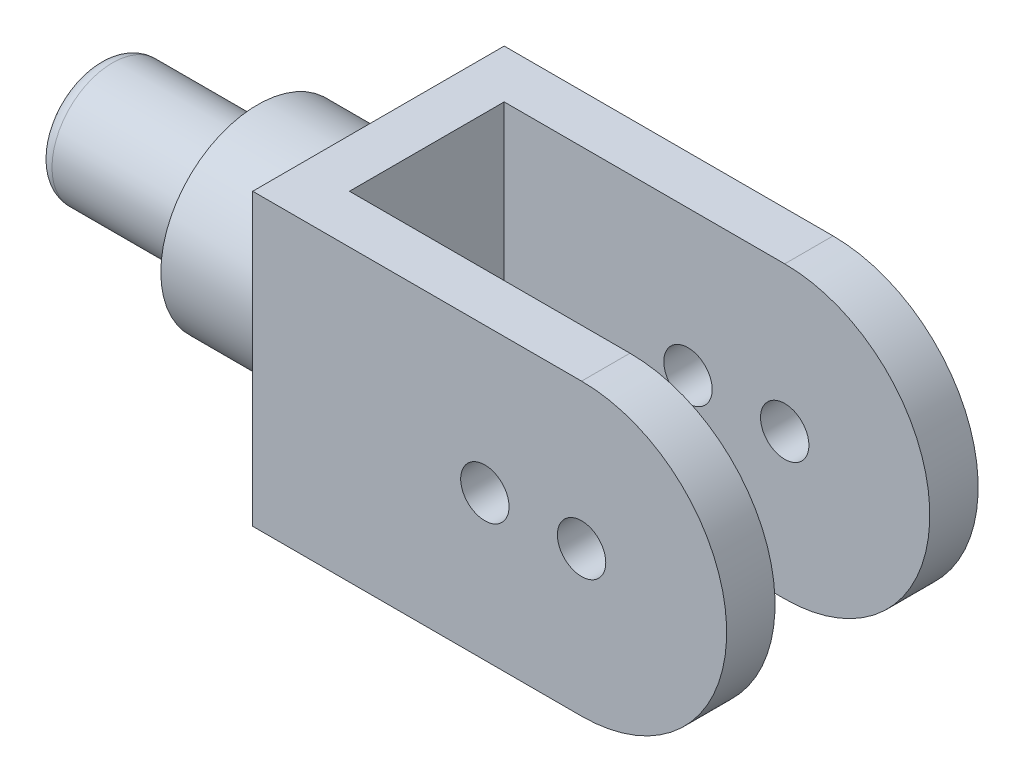
ISO-10303-21;
HEADER;
FILE_DESCRIPTION(('STEP AP214'),'2;1');
FILE_NAME('part.step','',(''),(''),'','','');
FILE_SCHEMA(('AUTOMOTIVE_DESIGN { 1 0 10303 214 1 1 1 1 }'));
ENDSEC;
DATA;
#1=APPLICATION_CONTEXT('core data for automotive mechanical design processes');
#2=APPLICATION_PROTOCOL_DEFINITION('international standard','automotive_design',2000,#1);
#3=PRODUCT_CONTEXT('',#1,'mechanical');
#4=PRODUCT('Part','Part','',(#3));
#5=PRODUCT_RELATED_PRODUCT_CATEGORY('part','',(#4));
#6=PRODUCT_DEFINITION_FORMATION('','',#4);
#7=PRODUCT_DEFINITION_CONTEXT('part definition',#1,'design');
#8=PRODUCT_DEFINITION('design','',#6,#7);
#9=PRODUCT_DEFINITION_SHAPE('','',#8);
#10=(LENGTH_UNIT() NAMED_UNIT(*) SI_UNIT(.MILLI.,.METRE.));
#11=(NAMED_UNIT(*) PLANE_ANGLE_UNIT() SI_UNIT($,.RADIAN.));
#12=(NAMED_UNIT(*) SI_UNIT($,.STERADIAN.) SOLID_ANGLE_UNIT());
#13=UNCERTAINTY_MEASURE_WITH_UNIT(LENGTH_MEASURE(1.E-05),#10,'distance_accuracy_value','');
#14=(GEOMETRIC_REPRESENTATION_CONTEXT(3) GLOBAL_UNCERTAINTY_ASSIGNED_CONTEXT((#13)) GLOBAL_UNIT_ASSIGNED_CONTEXT((#10,
#11,#12)) REPRESENTATION_CONTEXT('',''));
#15=CARTESIAN_POINT('',(0.,0.,0.));
#16=DIRECTION('',(0.,0.,1.));
#17=DIRECTION('',(1.,0.,0.));
#18=AXIS2_PLACEMENT_3D('',#15,#16,#17);
#19=CARTESIAN_POINT('',(10.,0.,0.));
#20=DIRECTION('',(1.,0.,0.));
#21=DIRECTION('',(0.,0.,-1.));
#22=AXIS2_PLACEMENT_3D('',#19,#20,#21);
#23=PLANE('',#22);
#24=DIRECTION('',(0.,0.,-1.));
#25=VECTOR('',#24,1.);
#26=CARTESIAN_POINT('',(10.,0.,0.));
#27=LINE('',#26,#25);
#28=CARTESIAN_POINT('',(10.,0.,0.));
#29=VERTEX_POINT('',#28);
#30=CARTESIAN_POINT('',(10.,0.,-32.));
#31=VERTEX_POINT('',#30);
#32=EDGE_CURVE('E53',#29,#31,#27,.T.);
#33=ORIENTED_EDGE('',*,*,#32,.T.);
#34=DIRECTION('',(0.,1.,0.));
#35=VECTOR('',#34,1.);
#36=CARTESIAN_POINT('',(9.99999999999999,60.,-32.));
#37=LINE('',#36,#35);
#38=CARTESIAN_POINT('',(10.,60.,-32.));
#39=VERTEX_POINT('',#38);
#40=EDGE_CURVE('E59',#31,#39,#37,.T.);
#41=ORIENTED_EDGE('',*,*,#40,.T.);
#42=DIRECTION('',(0.,0.,-1.));
#43=VECTOR('',#42,1.);
#44=CARTESIAN_POINT('',(10.,60.,0.));
#45=LINE('',#44,#43);
#46=CARTESIAN_POINT('',(10.,60.,0.));
#47=VERTEX_POINT('',#46);
#48=EDGE_CURVE('E123',#47,#39,#45,.T.);
#49=ORIENTED_EDGE('',*,*,#48,.F.);
#50=DIRECTION('',(0.,1.,0.));
#51=VECTOR('',#50,1.);
#52=CARTESIAN_POINT('',(10.,0.,0.));
#53=LINE('',#52,#51);
#54=EDGE_CURVE('E138',#29,#47,#53,.T.);
#55=ORIENTED_EDGE('',*,*,#54,.F.);
#56=EDGE_LOOP('',(#33,#41,#49,#55));
#57=FACE_BOUND('',#56,.T.);
#58=ADVANCED_FACE('F39',(#57),#23,.T.);
#59=CARTESIAN_POINT('',(68.,30.,0.));
#60=DIRECTION('',(0.,0.,-1.));
#61=DIRECTION('',(-1.,0.,0.));
#62=AXIS2_PLACEMENT_3D('',#59,#60,#61);
#63=PLANE('',#62);
#64=CARTESIAN_POINT('',(68.,30.,0.));
#65=DIRECTION('',(0.,0.,1.));
#66=DIRECTION('',(1.,0.,0.));
#67=AXIS2_PLACEMENT_3D('',#64,#65,#66);
#68=CIRCLE('',#67,5.00000000000001);
#69=CARTESIAN_POINT('',(73.,30.,0.));
#70=VERTEX_POINT('',#69);
#71=EDGE_CURVE('E151',#70,#70,#68,.T.);
#72=ORIENTED_EDGE('',*,*,#71,.T.);
#73=EDGE_LOOP('',(#72));
#74=FACE_BOUND('',#73,.T.);
#75=CARTESIAN_POINT('',(48.,30.,0.));
#76=DIRECTION('',(0.,0.,1.));
#77=DIRECTION('',(1.,0.,0.));
#78=AXIS2_PLACEMENT_3D('',#75,#76,#77);
#79=CIRCLE('',#78,5.);
#80=CARTESIAN_POINT('',(53.,30.,0.));
#81=VERTEX_POINT('',#80);
#82=EDGE_CURVE('E143',#81,#81,#79,.T.);
#83=ORIENTED_EDGE('',*,*,#82,.T.);
#84=EDGE_LOOP('',(#83));
#85=FACE_BOUND('',#84,.T.);
#86=DIRECTION('',(1.,0.,0.));
#87=VECTOR('',#86,1.);
#88=CARTESIAN_POINT('',(0.,0.,0.));
#89=LINE('',#88,#87);
#90=CARTESIAN_POINT('',(68.,0.,0.));
#91=VERTEX_POINT('',#90);
#92=EDGE_CURVE('E156',#29,#91,#89,.T.);
#93=ORIENTED_EDGE('',*,*,#92,.F.);
#94=ORIENTED_EDGE('',*,*,#54,.T.);
#95=DIRECTION('',(-1.,0.,0.));
#96=VECTOR('',#95,1.);
#97=CARTESIAN_POINT('',(68.,60.,0.));
#98=LINE('',#97,#96);
#99=CARTESIAN_POINT('',(68.,60.,0.));
#100=VERTEX_POINT('',#99);
#101=EDGE_CURVE('E165',#100,#47,#98,.T.);
#102=ORIENTED_EDGE('',*,*,#101,.F.);
#103=CARTESIAN_POINT('',(68.,30.,0.));
#104=DIRECTION('',(0.,0.,1.));
#105=DIRECTION('',(-1.,0.,0.));
#106=AXIS2_PLACEMENT_3D('',#103,#104,#105);
#107=CIRCLE('',#106,30.);
#108=EDGE_CURVE('E175',#91,#100,#107,.T.);
#109=ORIENTED_EDGE('',*,*,#108,.F.);
#110=EDGE_LOOP('',(#93,#94,#102,#109));
#111=FACE_BOUND('',#110,.T.);
#112=ADVANCED_FACE('F233',(#74,#85,#111),#63,.T.);
#113=CARTESIAN_POINT('',(68.,30.,10.));
#114=DIRECTION('',(0.,0.,-1.));
#115=DIRECTION('',(-1.,0.,0.));
#116=AXIS2_PLACEMENT_3D('',#113,#114,#115);
#117=PLANE('',#116);
#118=DIRECTION('',(0.,-1.,0.));
#119=VECTOR('',#118,1.);
#120=CARTESIAN_POINT('',(0.,60.,10.));
#121=LINE('',#120,#119);
#122=CARTESIAN_POINT('',(0.,60.,10.));
#123=VERTEX_POINT('',#122);
#124=CARTESIAN_POINT('',(0.,0.,10.));
#125=VERTEX_POINT('',#124);
#126=EDGE_CURVE('E157',#123,#125,#121,.T.);
#127=ORIENTED_EDGE('',*,*,#126,.T.);
#128=DIRECTION('',(1.,0.,0.));
#129=VECTOR('',#128,1.);
#130=CARTESIAN_POINT('',(0.,0.,10.));
#131=LINE('',#130,#129);
#132=CARTESIAN_POINT('',(68.,0.,10.));
#133=VERTEX_POINT('',#132);
#134=EDGE_CURVE('E161',#125,#133,#131,.T.);
#135=ORIENTED_EDGE('',*,*,#134,.T.);
#136=CARTESIAN_POINT('',(68.,30.,10.));
#137=DIRECTION('',(0.,0.,1.));
#138=DIRECTION('',(-1.,0.,0.));
#139=AXIS2_PLACEMENT_3D('',#136,#137,#138);
#140=CIRCLE('',#139,30.);
#141=CARTESIAN_POINT('',(68.,60.,10.));
#142=VERTEX_POINT('',#141);
#143=EDGE_CURVE('E168',#133,#142,#140,.T.);
#144=ORIENTED_EDGE('',*,*,#143,.T.);
#145=DIRECTION('',(-1.,0.,0.));
#146=VECTOR('',#145,1.);
#147=CARTESIAN_POINT('',(68.,60.,10.));
#148=LINE('',#147,#146);
#149=EDGE_CURVE('E166',#142,#123,#148,.T.);
#150=ORIENTED_EDGE('',*,*,#149,.T.);
#151=EDGE_LOOP('',(#127,#135,#144,#150));
#152=FACE_BOUND('',#151,.T.);
#153=CARTESIAN_POINT('',(68.,30.,10.));
#154=DIRECTION('',(0.,0.,1.));
#155=DIRECTION('',(1.,0.,0.));
#156=AXIS2_PLACEMENT_3D('',#153,#154,#155);
#157=CIRCLE('',#156,5.00000000000001);
#158=CARTESIAN_POINT('',(73.,30.,10.));
#159=VERTEX_POINT('',#158);
#160=EDGE_CURVE('E152',#159,#159,#157,.T.);
#161=ORIENTED_EDGE('',*,*,#160,.F.);
#162=EDGE_LOOP('',(#161));
#163=FACE_BOUND('',#162,.T.);
#164=CARTESIAN_POINT('',(48.,30.,10.));
#165=DIRECTION('',(0.,0.,1.));
#166=DIRECTION('',(1.,0.,0.));
#167=AXIS2_PLACEMENT_3D('',#164,#165,#166);
#168=CIRCLE('',#167,5.);
#169=CARTESIAN_POINT('',(53.,30.,10.));
#170=VERTEX_POINT('',#169);
#171=EDGE_CURVE('E149',#170,#170,#168,.T.);
#172=ORIENTED_EDGE('',*,*,#171,.F.);
#173=EDGE_LOOP('',(#172));
#174=FACE_BOUND('',#173,.T.);
#175=ADVANCED_FACE('F236',(#152,#163,#174),#117,.F.);
#176=CARTESIAN_POINT('',(0.,60.,10.));
#177=DIRECTION('',(1.,0.,0.));
#178=DIRECTION('',(0.,0.,-1.));
#179=AXIS2_PLACEMENT_3D('',#176,#177,#178);
#180=PLANE('',#179);
#181=CARTESIAN_POINT('',(0.,30.,-16.));
#182=DIRECTION('',(1.,0.,0.));
#183=DIRECTION('',(0.,0.,-1.));
#184=AXIS2_PLACEMENT_3D('',#181,#182,#183);
#185=CIRCLE('',#184,23.);
#186=CARTESIAN_POINT('',(0.,30.,-39.));
#187=VERTEX_POINT('',#186);
#188=EDGE_CURVE('E190',#187,#187,#185,.T.);
#189=ORIENTED_EDGE('',*,*,#188,.T.);
#190=EDGE_LOOP('',(#189));
#191=FACE_BOUND('',#190,.T.);
#192=DIRECTION('',(0.,0.,-1.));
#193=VECTOR('',#192,1.);
#194=CARTESIAN_POINT('',(0.,60.,10.));
#195=LINE('',#194,#193);
#196=CARTESIAN_POINT('',(0.,60.,-42.));
#197=VERTEX_POINT('',#196);
#198=EDGE_CURVE('E167',#123,#197,#195,.T.);
#199=ORIENTED_EDGE('',*,*,#198,.T.);
#200=DIRECTION('',(0.,1.,0.));
#201=VECTOR('',#200,1.);
#202=CARTESIAN_POINT('',(0.,0.,-42.));
#203=LINE('',#202,#201);
#204=CARTESIAN_POINT('',(0.,0.,-42.));
#205=VERTEX_POINT('',#204);
#206=EDGE_CURVE('E145',#205,#197,#203,.T.);
#207=ORIENTED_EDGE('',*,*,#206,.F.);
#208=DIRECTION('',(0.,0.,-1.));
#209=VECTOR('',#208,1.);
#210=CARTESIAN_POINT('',(0.,0.,10.));
#211=LINE('',#210,#209);
#212=EDGE_CURVE('E185',#125,#205,#211,.T.);
#213=ORIENTED_EDGE('',*,*,#212,.F.);
#214=ORIENTED_EDGE('',*,*,#126,.F.);
#215=EDGE_LOOP('',(#199,#207,#213,#214));
#216=FACE_BOUND('',#215,.T.);
#217=ADVANCED_FACE('F242',(#191,#216),#180,.F.);
#218=CARTESIAN_POINT('',(0.,0.,10.));
#219=DIRECTION('',(0.,1.,0.));
#220=DIRECTION('',(0.,0.,1.));
#221=AXIS2_PLACEMENT_3D('',#218,#219,#220);
#222=PLANE('',#221);
#223=ORIENTED_EDGE('',*,*,#212,.T.);
#224=DIRECTION('',(-1.,0.,0.));
#225=VECTOR('',#224,1.);
#226=CARTESIAN_POINT('',(0.,0.,-42.));
#227=LINE('',#226,#225);
#228=CARTESIAN_POINT('',(68.0000000000001,0.,-41.9999999999999));
#229=VERTEX_POINT('',#228);
#230=EDGE_CURVE('E134',#229,#205,#227,.T.);
#231=ORIENTED_EDGE('',*,*,#230,.F.);
#232=DIRECTION('',(0.,0.,-1.));
#233=VECTOR('',#232,1.);
#234=CARTESIAN_POINT('',(68.0000000000001,0.,-31.9999999999999));
#235=LINE('',#234,#233);
#236=CARTESIAN_POINT('',(68.0000000000001,0.,-31.9999999999999));
#237=VERTEX_POINT('',#236);
#238=EDGE_CURVE('E112',#237,#229,#235,.T.);
#239=ORIENTED_EDGE('',*,*,#238,.F.);
#240=DIRECTION('',(-1.,0.,0.));
#241=VECTOR('',#240,1.);
#242=CARTESIAN_POINT('',(9.99999999999999,0.,-32.));
#243=LINE('',#242,#241);
#244=EDGE_CURVE('E114',#237,#31,#243,.T.);
#245=ORIENTED_EDGE('',*,*,#244,.T.);
#246=ORIENTED_EDGE('',*,*,#32,.F.);
#247=ORIENTED_EDGE('',*,*,#92,.T.);
#248=DIRECTION('',(0.,0.,-1.));
#249=VECTOR('',#248,1.);
#250=CARTESIAN_POINT('',(68.,0.,10.));
#251=LINE('',#250,#249);
#252=EDGE_CURVE('E177',#133,#91,#251,.T.);
#253=ORIENTED_EDGE('',*,*,#252,.F.);
#254=ORIENTED_EDGE('',*,*,#134,.F.);
#255=EDGE_LOOP('',(#223,#231,#239,#245,#246,#247,#253,#254));
#256=FACE_BOUND('',#255,.T.);
#257=ADVANCED_FACE('F252',(#256),#222,.F.);
#258=CARTESIAN_POINT('',(68.,30.,10.));
#259=DIRECTION('',(0.,0.,-1.));
#260=DIRECTION('',(-1.,0.,0.));
#261=AXIS2_PLACEMENT_3D('',#258,#259,#260);
#262=CYLINDRICAL_SURFACE('',#261,30.);
#263=ORIENTED_EDGE('',*,*,#108,.T.);
#264=DIRECTION('',(0.,0.,-1.));
#265=VECTOR('',#264,1.);
#266=CARTESIAN_POINT('',(68.,60.,10.));
#267=LINE('',#266,#265);
#268=EDGE_CURVE('E176',#142,#100,#267,.T.);
#269=ORIENTED_EDGE('',*,*,#268,.F.);
#270=ORIENTED_EDGE('',*,*,#143,.F.);
#271=ORIENTED_EDGE('',*,*,#252,.T.);
#272=EDGE_LOOP('',(#263,#269,#270,#271));
#273=FACE_BOUND('',#272,.T.);
#274=ADVANCED_FACE('F247',(#273),#262,.T.);
#275=CARTESIAN_POINT('',(68.,60.,10.));
#276=DIRECTION('',(0.,-1.,0.));
#277=DIRECTION('',(0.,0.,-1.));
#278=AXIS2_PLACEMENT_3D('',#275,#276,#277);
#279=PLANE('',#278);
#280=ORIENTED_EDGE('',*,*,#101,.T.);
#281=ORIENTED_EDGE('',*,*,#48,.T.);
#282=DIRECTION('',(1.,0.,0.));
#283=VECTOR('',#282,1.);
#284=CARTESIAN_POINT('',(9.99999999999999,60.,-32.));
#285=LINE('',#284,#283);
#286=CARTESIAN_POINT('',(68.,60.,-31.9999999999999));
#287=VERTEX_POINT('',#286);
#288=EDGE_CURVE('E119',#39,#287,#285,.T.);
#289=ORIENTED_EDGE('',*,*,#288,.T.);
#290=DIRECTION('',(0.,0.,-1.));
#291=VECTOR('',#290,1.);
#292=CARTESIAN_POINT('',(68.,60.,-31.9999999999999));
#293=LINE('',#292,#291);
#294=CARTESIAN_POINT('',(68.0000000000001,60.,-41.9999999999999));
#295=VERTEX_POINT('',#294);
#296=EDGE_CURVE('E101',#287,#295,#293,.T.);
#297=ORIENTED_EDGE('',*,*,#296,.T.);
#298=DIRECTION('',(-1.,0.,0.));
#299=VECTOR('',#298,1.);
#300=CARTESIAN_POINT('',(0.,60.,-42.));
#301=LINE('',#300,#299);
#302=EDGE_CURVE('E139',#295,#197,#301,.T.);
#303=ORIENTED_EDGE('',*,*,#302,.T.);
#304=ORIENTED_EDGE('',*,*,#198,.F.);
#305=ORIENTED_EDGE('',*,*,#149,.F.);
#306=ORIENTED_EDGE('',*,*,#268,.T.);
#307=EDGE_LOOP('',(#280,#281,#289,#297,#303,#304,#305,#306));
#308=FACE_BOUND('',#307,.T.);
#309=ADVANCED_FACE('F121',(#308),#279,.F.);
#310=CARTESIAN_POINT('',(68.,30.,10.));
#311=DIRECTION('',(0.,0.,-1.));
#312=DIRECTION('',(-1.,0.,0.));
#313=AXIS2_PLACEMENT_3D('',#310,#311,#312);
#314=CYLINDRICAL_SURFACE('',#313,5.00000000000001);
#315=ORIENTED_EDGE('',*,*,#160,.T.);
#316=EDGE_LOOP('',(#315));
#317=FACE_BOUND('',#316,.T.);
#318=ORIENTED_EDGE('',*,*,#71,.F.);
#319=EDGE_LOOP('',(#318));
#320=FACE_BOUND('',#319,.T.);
#321=ADVANCED_FACE('F222',(#317,#320),#314,.F.);
#322=CARTESIAN_POINT('',(48.,30.,10.));
#323=DIRECTION('',(0.,0.,-1.));
#324=DIRECTION('',(-1.,0.,0.));
#325=AXIS2_PLACEMENT_3D('',#322,#323,#324);
#326=CYLINDRICAL_SURFACE('',#325,5.);
#327=ORIENTED_EDGE('',*,*,#171,.T.);
#328=EDGE_LOOP('',(#327));
#329=FACE_BOUND('',#328,.T.);
#330=ORIENTED_EDGE('',*,*,#82,.F.);
#331=EDGE_LOOP('',(#330));
#332=FACE_BOUND('',#331,.T.);
#333=ADVANCED_FACE('F216',(#329,#332),#326,.F.);
#334=CARTESIAN_POINT('',(0.,0.,-42.));
#335=DIRECTION('',(0.,0.,-1.));
#336=DIRECTION('',(-1.,0.,0.));
#337=AXIS2_PLACEMENT_3D('',#334,#335,#336);
#338=PLANE('',#337);
#339=ORIENTED_EDGE('',*,*,#302,.F.);
#340=CARTESIAN_POINT('',(68.,30.,-41.9999999999999));
#341=DIRECTION('',(0.,0.,-1.));
#342=DIRECTION('',(-1.,0.,0.));
#343=AXIS2_PLACEMENT_3D('',#340,#341,#342);
#344=CIRCLE('',#343,30.);
#345=EDGE_CURVE('E109',#295,#229,#344,.T.);
#346=ORIENTED_EDGE('',*,*,#345,.T.);
#347=ORIENTED_EDGE('',*,*,#230,.T.);
#348=ORIENTED_EDGE('',*,*,#206,.T.);
#349=EDGE_LOOP('',(#339,#346,#347,#348));
#350=FACE_BOUND('',#349,.T.);
#351=CARTESIAN_POINT('',(48.0000000000001,30.,-41.9999999999999));
#352=DIRECTION('',(0.,0.,-1.));
#353=DIRECTION('',(-1.,0.,0.));
#354=AXIS2_PLACEMENT_3D('',#351,#352,#353);
#355=CIRCLE('',#354,5.);
#356=CARTESIAN_POINT('',(43.0000000000001,30.,-41.9999999999999));
#357=VERTEX_POINT('',#356);
#358=EDGE_CURVE('E204',#357,#357,#355,.T.);
#359=ORIENTED_EDGE('',*,*,#358,.F.);
#360=EDGE_LOOP('',(#359));
#361=FACE_BOUND('',#360,.T.);
#362=CARTESIAN_POINT('',(68.,30.,-41.9999999999999));
#363=DIRECTION('',(0.,0.,-1.));
#364=DIRECTION('',(-1.,0.,0.));
#365=AXIS2_PLACEMENT_3D('',#362,#363,#364);
#366=CIRCLE('',#365,4.99999999999998);
#367=CARTESIAN_POINT('',(63.,30.,-41.9999999999999));
#368=VERTEX_POINT('',#367);
#369=EDGE_CURVE('E202',#368,#368,#366,.T.);
#370=ORIENTED_EDGE('',*,*,#369,.F.);
#371=EDGE_LOOP('',(#370));
#372=FACE_BOUND('',#371,.T.);
#373=ADVANCED_FACE('F211',(#350,#361,#372),#338,.T.);
#374=CARTESIAN_POINT('',(68.,30.,-31.9999999999999));
#375=DIRECTION('',(0.,0.,-1.));
#376=DIRECTION('',(-1.,0.,0.));
#377=AXIS2_PLACEMENT_3D('',#374,#375,#376);
#378=CYLINDRICAL_SURFACE('',#377,30.);
#379=ORIENTED_EDGE('',*,*,#345,.F.);
#380=ORIENTED_EDGE('',*,*,#296,.F.);
#381=CARTESIAN_POINT('',(68.,30.,-31.9999999999999));
#382=DIRECTION('',(0.,0.,-1.));
#383=DIRECTION('',(-1.,0.,0.));
#384=AXIS2_PLACEMENT_3D('',#381,#382,#383);
#385=CIRCLE('',#384,30.);
#386=EDGE_CURVE('E110',#287,#237,#385,.T.);
#387=ORIENTED_EDGE('',*,*,#386,.T.);
#388=ORIENTED_EDGE('',*,*,#238,.T.);
#389=EDGE_LOOP('',(#379,#380,#387,#388));
#390=FACE_BOUND('',#389,.T.);
#391=ADVANCED_FACE('F102',(#390),#378,.T.);
#392=CARTESIAN_POINT('',(68.,30.,-31.9999999999999));
#393=DIRECTION('',(0.,0.,-1.));
#394=DIRECTION('',(-1.,0.,0.));
#395=AXIS2_PLACEMENT_3D('',#392,#393,#394);
#396=PLANE('',#395);
#397=CARTESIAN_POINT('',(48.,30.,-31.9999999999999));
#398=DIRECTION('',(0.,0.,-1.));
#399=DIRECTION('',(-1.,0.,0.));
#400=AXIS2_PLACEMENT_3D('',#397,#398,#399);
#401=CIRCLE('',#400,5.);
#402=CARTESIAN_POINT('',(43.,30.,-31.9999999999999));
#403=VERTEX_POINT('',#402);
#404=EDGE_CURVE('E201',#403,#403,#401,.T.);
#405=ORIENTED_EDGE('',*,*,#404,.T.);
#406=EDGE_LOOP('',(#405));
#407=FACE_BOUND('',#406,.T.);
#408=CARTESIAN_POINT('',(68.,30.,-31.9999999999999));
#409=DIRECTION('',(0.,0.,-1.));
#410=DIRECTION('',(-1.,0.,0.));
#411=AXIS2_PLACEMENT_3D('',#408,#409,#410);
#412=CIRCLE('',#411,4.99999999999998);
#413=CARTESIAN_POINT('',(63.,30.,-31.9999999999999));
#414=VERTEX_POINT('',#413);
#415=EDGE_CURVE('E135',#414,#414,#412,.T.);
#416=ORIENTED_EDGE('',*,*,#415,.T.);
#417=EDGE_LOOP('',(#416));
#418=FACE_BOUND('',#417,.T.);
#419=ORIENTED_EDGE('',*,*,#40,.F.);
#420=ORIENTED_EDGE('',*,*,#244,.F.);
#421=ORIENTED_EDGE('',*,*,#386,.F.);
#422=ORIENTED_EDGE('',*,*,#288,.F.);
#423=EDGE_LOOP('',(#419,#420,#421,#422));
#424=FACE_BOUND('',#423,.T.);
#425=ADVANCED_FACE('F118',(#407,#418,#424),#396,.F.);
#426=CARTESIAN_POINT('',(68.,30.,-31.9999999999999));
#427=DIRECTION('',(0.,0.,-1.));
#428=DIRECTION('',(-1.,0.,0.));
#429=AXIS2_PLACEMENT_3D('',#426,#427,#428);
#430=CYLINDRICAL_SURFACE('',#429,4.99999999999998);
#431=ORIENTED_EDGE('',*,*,#415,.F.);
#432=EDGE_LOOP('',(#431));
#433=FACE_BOUND('',#432,.T.);
#434=ORIENTED_EDGE('',*,*,#369,.T.);
#435=EDGE_LOOP('',(#434));
#436=FACE_BOUND('',#435,.T.);
#437=ADVANCED_FACE('F215',(#433,#436),#430,.F.);
#438=CARTESIAN_POINT('',(48.,30.,-31.9999999999999));
#439=DIRECTION('',(0.,0.,-1.));
#440=DIRECTION('',(-1.,0.,0.));
#441=AXIS2_PLACEMENT_3D('',#438,#439,#440);
#442=CYLINDRICAL_SURFACE('',#441,5.);
#443=ORIENTED_EDGE('',*,*,#404,.F.);
#444=EDGE_LOOP('',(#443));
#445=FACE_BOUND('',#444,.T.);
#446=ORIENTED_EDGE('',*,*,#358,.T.);
#447=EDGE_LOOP('',(#446));
#448=FACE_BOUND('',#447,.T.);
#449=ADVANCED_FACE('F279',(#445,#448),#442,.F.);
#450=CARTESIAN_POINT('',(-25.,30.,-16.));
#451=DIRECTION('',(1.,0.,0.));
#452=DIRECTION('',(0.,0.,-1.));
#453=AXIS2_PLACEMENT_3D('',#450,#451,#452);
#454=CYLINDRICAL_SURFACE('',#453,20.);
#455=CARTESIAN_POINT('',(-3.,30.,-16.));
#456=DIRECTION('',(1.,0.,0.));
#457=DIRECTION('',(0.,0.,-1.));
#458=AXIS2_PLACEMENT_3D('',#455,#456,#457);
#459=CIRCLE('',#458,20.);
#460=CARTESIAN_POINT('',(-3.,30.,-36.));
#461=VERTEX_POINT('',#460);
#462=EDGE_CURVE('E183',#461,#461,#459,.F.);
#463=ORIENTED_EDGE('',*,*,#462,.T.);
#464=EDGE_LOOP('',(#463));
#465=FACE_BOUND('',#464,.T.);
#466=CARTESIAN_POINT('',(-25.,30.,-16.));
#467=DIRECTION('',(-1.,0.,0.));
#468=DIRECTION('',(0.,0.,1.));
#469=AXIS2_PLACEMENT_3D('',#466,#467,#468);
#470=CIRCLE('',#469,20.);
#471=CARTESIAN_POINT('',(-25.,30.,4.));
#472=VERTEX_POINT('',#471);
#473=EDGE_CURVE('E198',#472,#472,#470,.T.);
#474=ORIENTED_EDGE('',*,*,#473,.F.);
#475=EDGE_LOOP('',(#474));
#476=FACE_BOUND('',#475,.T.);
#477=ADVANCED_FACE('F267',(#465,#476),#454,.T.);
#478=CARTESIAN_POINT('',(-25.,30.,-16.));
#479=DIRECTION('',(-1.,0.,0.));
#480=DIRECTION('',(0.,0.,1.));
#481=AXIS2_PLACEMENT_3D('',#478,#479,#480);
#482=PLANE('',#481);
#483=CARTESIAN_POINT('',(-25.,30.,-16.));
#484=DIRECTION('',(-1.,0.,0.));
#485=DIRECTION('',(0.,0.,1.));
#486=AXIS2_PLACEMENT_3D('',#483,#484,#485);
#487=CIRCLE('',#486,12.5);
#488=CARTESIAN_POINT('',(-25.,30.,-3.5));
#489=VERTEX_POINT('',#488);
#490=EDGE_CURVE('E186',#489,#489,#487,.T.);
#491=ORIENTED_EDGE('',*,*,#490,.F.);
#492=EDGE_LOOP('',(#491));
#493=FACE_BOUND('',#492,.T.);
#494=ORIENTED_EDGE('',*,*,#473,.T.);
#495=EDGE_LOOP('',(#494));
#496=FACE_BOUND('',#495,.T.);
#497=ADVANCED_FACE('F258',(#493,#496),#482,.T.);
#498=CARTESIAN_POINT('',(-3.,30.,-16.));
#499=DIRECTION('',(1.,0.,0.));
#500=DIRECTION('',(0.,0.,-1.));
#501=AXIS2_PLACEMENT_3D('',#498,#499,#500);
#502=TOROIDAL_SURFACE('',#501,23.,3.);
#503=ORIENTED_EDGE('',*,*,#188,.F.);
#504=EDGE_LOOP('',(#503));
#505=FACE_BOUND('',#504,.T.);
#506=ORIENTED_EDGE('',*,*,#462,.F.);
#507=EDGE_LOOP('',(#506));
#508=FACE_BOUND('',#507,.T.);
#509=ADVANCED_FACE('F260',(#505,#508),#502,.F.);
#510=CARTESIAN_POINT('',(-58.,30.,-16.));
#511=DIRECTION('',(1.,0.,0.));
#512=DIRECTION('',(0.,0.,-1.));
#513=AXIS2_PLACEMENT_3D('',#510,#511,#512);
#514=CYLINDRICAL_SURFACE('',#513,12.5);
#515=CARTESIAN_POINT('',(-55.,30.,-16.));
#516=DIRECTION('',(-1.,0.,0.));
#517=DIRECTION('',(0.,0.,1.));
#518=AXIS2_PLACEMENT_3D('',#515,#516,#517);
#519=CIRCLE('',#518,12.5);
#520=CARTESIAN_POINT('',(-55.,30.,-3.5));
#521=VERTEX_POINT('',#520);
#522=EDGE_CURVE('E11',#521,#521,#519,.F.);
#523=ORIENTED_EDGE('',*,*,#522,.T.);
#524=EDGE_LOOP('',(#523));
#525=FACE_BOUND('',#524,.T.);
#526=ORIENTED_EDGE('',*,*,#490,.T.);
#527=EDGE_LOOP('',(#526));
#528=FACE_BOUND('',#527,.T.);
#529=ADVANCED_FACE('F256',(#525,#528),#514,.T.);
#530=CARTESIAN_POINT('',(-58.,30.,-16.));
#531=DIRECTION('',(-1.,0.,0.));
#532=DIRECTION('',(0.,0.,1.));
#533=AXIS2_PLACEMENT_3D('',#530,#531,#532);
#534=PLANE('',#533);
#535=CARTESIAN_POINT('',(-58.,30.,-16.));
#536=DIRECTION('',(-1.,0.,0.));
#537=DIRECTION('',(0.,0.,1.));
#538=AXIS2_PLACEMENT_3D('',#535,#536,#537);
#539=CIRCLE('',#538,9.5);
#540=CARTESIAN_POINT('',(-58.,30.,-6.5));
#541=VERTEX_POINT('',#540);
#542=EDGE_CURVE('E50',#541,#541,#539,.T.);
#543=ORIENTED_EDGE('',*,*,#542,.T.);
#544=EDGE_LOOP('',(#543));
#545=FACE_BOUND('',#544,.T.);
#546=ADVANCED_FACE('F266',(#545),#534,.T.);
#547=CARTESIAN_POINT('',(-55.,30.,-16.));
#548=DIRECTION('',(-1.,0.,0.));
#549=DIRECTION('',(0.,0.,1.));
#550=AXIS2_PLACEMENT_3D('',#547,#548,#549);
#551=TOROIDAL_SURFACE('',#550,9.5,3.);
#552=ORIENTED_EDGE('',*,*,#522,.F.);
#553=EDGE_LOOP('',(#552));
#554=FACE_BOUND('',#553,.T.);
#555=ORIENTED_EDGE('',*,*,#542,.F.);
#556=EDGE_LOOP('',(#555));
#557=FACE_BOUND('',#556,.T.);
#558=ADVANCED_FACE('F41',(#554,#557),#551,.T.);
#559=CLOSED_SHELL('',(#58,#112,#175,#217,#257,#274,#309,#321,#333,#373,#391,#425,#437,#449,#477,
#497,#509,#529,#546,#558));
#560=MANIFOLD_SOLID_BREP('B2',#559);
#561=ADVANCED_BREP_SHAPE_REPRESENTATION('',(#18,#560),#14);
#562=SHAPE_DEFINITION_REPRESENTATION(#9,#561);
ENDSEC;
END-ISO-10303-21;
